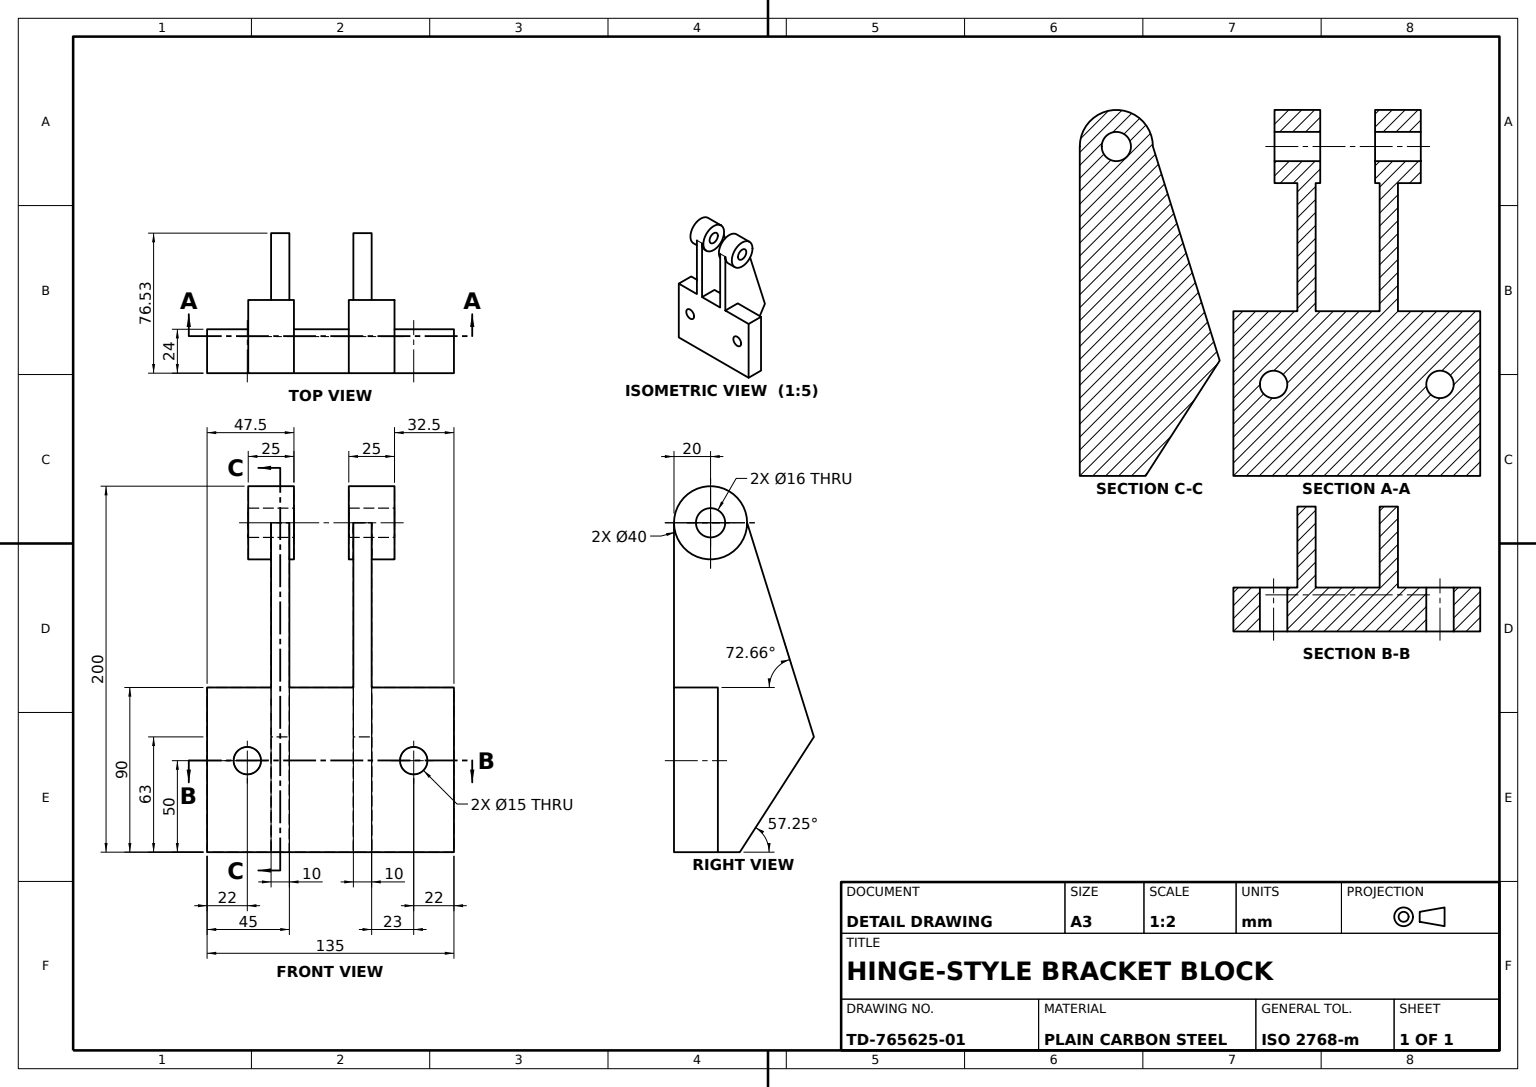
SolidWorks part; units mm, degrees
material "Plain Carbon Steel"
ref_plane "Front Plane" through (0, 0, 0) normal (0, 0, 1) x (1, 0, 0)
ref_plane "Top Plane" through (0, 0, 0) normal (0, 1, 0) x (1, 0, 0)
ref_plane "Right Plane" through (0, 0, 0) normal (1, 0, 0) x (0, 0, -1)
sketch "Base Plate Sketch" plane through (0, 0, 0) normal (0, 0, 1) x (1, 0, 0)
  line L0 (0, 0) -> (0, 90)
  line L1 (0, 90) -> (135, 90)
  line L2 (135, 90) -> (135, 0)
  line L3 (135, 0) -> (0, 0)
  dimension "D1" = 90
  dimension "D2" = 135
extrude "Base Plate" add sketch "Base Plate Sketch" against normal blind 24
ref_plane "Lug 1 Plane" through (90, 0, 0) normal (1, 0, 0) x (0, 0, -1)
sketch "Lug 1 Profile" plane through (90, 0, 0) normal (1, 0, 0) x (0, 0, -1)
  line L0 (0, 90) -> (0, 180)
  line L2 (0, 90) -> (24, 90)
  line L3 (24, 90) -> (24, 0)
  line L4 (24, 0) -> (36, 0)
  line L5 (36, 0) -> (76.5257, 63)
  line L6 (76.5257, 63) -> (40, 180)
  arc A0 (0, 180) -> (40, 180) centre (20, 180) ccw
  dimension "D3" = 12
  dimension "D1" = 90
  dimension "D2" = 20
  dimension "D4" = 63
  dimension "D5" = 17.338
extrude "Lug 1" add sketch "Lug 1 Profile" against normal blind 10
sketch "Lug 1 Boss Sketch" plane through (90, 0, 0) normal (1, 0, 0) x (0, 0, -1)
  circle A0 centre (20, 180) radius 20
extrude "Lug 1 Pivot Boss" add sketch "Lug 1 Boss Sketch" along normal mid plane 25
ref_plane "Lug 2 Plane" through (45, 0, 0) normal (-1, 0, 0) x (0, 0, 1)
sketch "Lug 2 Profile" plane through (45, 0, 0) normal (-1, 0, 0) x (0, 0, 1)
  line L0 (-24, 0) -> (-36, 0)
  line L1 (-36, 0) -> (-76.5257, 63)
  line L2 (-76.5257, 63) -> (-40, 180)
  line L3 (0, 180) -> (0, 90)
  line L4 (0, 90) -> (-24, 90)
  line L5 (-24, 90) -> (-24, 0)
  arc A0 (-40, 180) -> (0, 180) centre (-20, 180) ccw
extrude "Lug 2" add sketch "Lug 2 Profile" along normal blind 10
sketch "Lug 2 Boss Sketch" plane through (35, 0, 0) normal (-1, 0, 0) x (0, 0, 1)
  circle A0 centre (-20, 180) radius 20
extrude "Lug 2 Pivot Boss" add sketch "Lug 2 Boss Sketch" along normal mid plane 25
sketch "Pivot Hole Sketch" plane through (102.5, 0, 0) normal (1, 0, 0) x (0, 0, -1)
  circle A0 centre (20, 180) radius 8
  dimension "D1" = 16
extrude "Pivot Hole Ø16" cut sketch "Pivot Hole Sketch" against normal through all
sketch "Mounting Holes Sketch" plane through (0, 0, -24) normal (0, 0, -1) x (-1, 0, 0)
  line L0 (-135, 90) -> (-90, 90) construction
  line L1 (-135, 0) -> (-135, 90) construction
  line L2 (0, 90) -> (0, 0) construction
  line L3 (-35, 90) -> (0, 90) construction
  circle A0 centre (-113, 50) radius 7.5
  circle A1 centre (-22, 50) radius 7.5
  dimension "D1" = 15
  dimension "D5" = 15
  dimension "D2" = 40
  dimension "D3" = 22
  dimension "D4" = 22
  dimension "D6" = 40
extrude "Mounting Holes 2x" cut sketch "Mounting Holes Sketch" against normal through all
